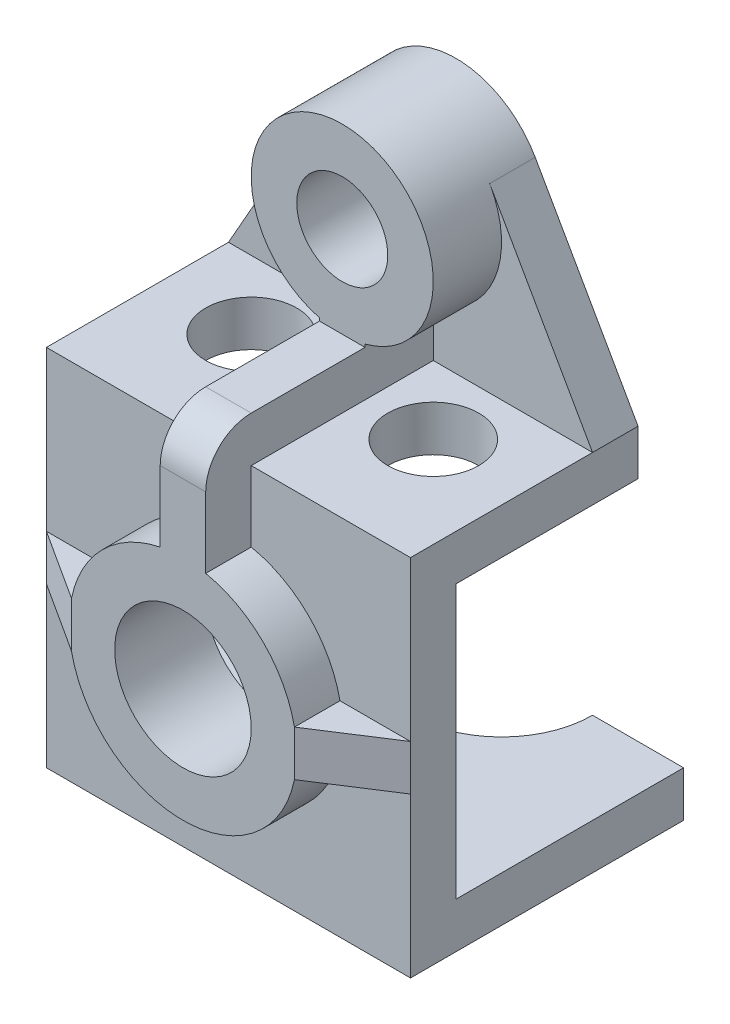
ISO-10303-21;
HEADER;
FILE_DESCRIPTION(('STEP AP214'),'2;1');
FILE_NAME('part.step','',(''),(''),'','','');
FILE_SCHEMA(('AUTOMOTIVE_DESIGN { 1 0 10303 214 1 1 1 1 }'));
ENDSEC;
DATA;
#1=APPLICATION_CONTEXT('core data for automotive mechanical design processes');
#2=APPLICATION_PROTOCOL_DEFINITION('international standard','automotive_design',2000,#1);
#3=PRODUCT_CONTEXT('',#1,'mechanical');
#4=PRODUCT('Part','Part','',(#3));
#5=PRODUCT_RELATED_PRODUCT_CATEGORY('part','',(#4));
#6=PRODUCT_DEFINITION_FORMATION('','',#4);
#7=PRODUCT_DEFINITION_CONTEXT('part definition',#1,'design');
#8=PRODUCT_DEFINITION('design','',#6,#7);
#9=PRODUCT_DEFINITION_SHAPE('','',#8);
#10=(LENGTH_UNIT() NAMED_UNIT(*) SI_UNIT(.MILLI.,.METRE.));
#11=(NAMED_UNIT(*) PLANE_ANGLE_UNIT() SI_UNIT($,.RADIAN.));
#12=(NAMED_UNIT(*) SI_UNIT($,.STERADIAN.) SOLID_ANGLE_UNIT());
#13=UNCERTAINTY_MEASURE_WITH_UNIT(LENGTH_MEASURE(1.E-05),#10,'distance_accuracy_value','');
#14=(GEOMETRIC_REPRESENTATION_CONTEXT(3) GLOBAL_UNCERTAINTY_ASSIGNED_CONTEXT((#13)) GLOBAL_UNIT_ASSIGNED_CONTEXT((#10,
#11,#12)) REPRESENTATION_CONTEXT('',''));
#15=CARTESIAN_POINT('',(0.,0.,0.));
#16=DIRECTION('',(0.,0.,1.));
#17=DIRECTION('',(1.,0.,0.));
#18=AXIS2_PLACEMENT_3D('',#15,#16,#17);
#19=CARTESIAN_POINT('',(40.,0.,-60.));
#20=DIRECTION('',(0.,0.,1.));
#21=DIRECTION('',(1.,0.,0.));
#22=AXIS2_PLACEMENT_3D('',#19,#20,#21);
#23=PLANE('',#22);
#24=DIRECTION('',(0.,1.,0.));
#25=VECTOR('',#24,1.);
#26=CARTESIAN_POINT('',(20.,-0.000999999999999265,-60.));
#27=LINE('',#26,#25);
#28=CARTESIAN_POINT('',(20.,10.,-60.));
#29=VERTEX_POINT('',#28);
#30=CARTESIAN_POINT('',(20.,0.,-60.));
#31=VERTEX_POINT('',#30);
#32=EDGE_CURVE('E226',#29,#31,#27,.F.);
#33=ORIENTED_EDGE('',*,*,#32,.F.);
#34=DIRECTION('',(-1.,0.,0.));
#35=VECTOR('',#34,1.);
#36=CARTESIAN_POINT('',(40.,10.,-60.));
#37=LINE('',#36,#35);
#38=CARTESIAN_POINT('',(40.,10.,-60.));
#39=VERTEX_POINT('',#38);
#40=EDGE_CURVE('E237',#39,#29,#37,.T.);
#41=ORIENTED_EDGE('',*,*,#40,.F.);
#42=DIRECTION('',(0.,1.,0.));
#43=VECTOR('',#42,1.);
#44=CARTESIAN_POINT('',(40.,0.,-60.));
#45=LINE('',#44,#43);
#46=CARTESIAN_POINT('',(40.,0.,-60.));
#47=VERTEX_POINT('',#46);
#48=EDGE_CURVE('E388',#47,#39,#45,.T.);
#49=ORIENTED_EDGE('',*,*,#48,.F.);
#50=DIRECTION('',(-1.,0.,0.));
#51=VECTOR('',#50,1.);
#52=CARTESIAN_POINT('',(40.,0.,-60.));
#53=LINE('',#52,#51);
#54=EDGE_CURVE('E245',#47,#31,#53,.T.);
#55=ORIENTED_EDGE('',*,*,#54,.T.);
#56=EDGE_LOOP('',(#33,#41,#49,#55));
#57=FACE_BOUND('',#56,.T.);
#58=ADVANCED_FACE('F43',(#57),#23,.F.);
#59=DIRECTION('',(0.,1.,0.));
#60=VECTOR('',#59,1.);
#61=CARTESIAN_POINT('',(-20.,-0.000999999999999265,-60.));
#62=LINE('',#61,#60);
#63=CARTESIAN_POINT('',(-20.,0.,-60.));
#64=VERTEX_POINT('',#63);
#65=CARTESIAN_POINT('',(-20.,10.,-60.));
#66=VERTEX_POINT('',#65);
#67=EDGE_CURVE('E59',#64,#66,#62,.T.);
#68=ORIENTED_EDGE('',*,*,#67,.F.);
#69=CARTESIAN_POINT('',(-40.,0.,-60.));
#70=VERTEX_POINT('',#69);
#71=EDGE_CURVE('E250',#64,#70,#53,.T.);
#72=ORIENTED_EDGE('',*,*,#71,.T.);
#73=DIRECTION('',(0.,1.,0.));
#74=VECTOR('',#73,1.);
#75=CARTESIAN_POINT('',(-40.,0.,-60.));
#76=LINE('',#75,#74);
#77=CARTESIAN_POINT('',(-40.,10.,-60.));
#78=VERTEX_POINT('',#77);
#79=EDGE_CURVE('E408',#70,#78,#76,.T.);
#80=ORIENTED_EDGE('',*,*,#79,.T.);
#81=EDGE_CURVE('E247',#66,#78,#37,.T.);
#82=ORIENTED_EDGE('',*,*,#81,.F.);
#83=EDGE_LOOP('',(#68,#72,#80,#82));
#84=FACE_BOUND('',#83,.T.);
#85=ADVANCED_FACE('F588',(#84),#23,.F.);
#86=CARTESIAN_POINT('',(40.,0.,0.));
#87=DIRECTION('',(0.,1.,0.));
#88=DIRECTION('',(0.,0.,1.));
#89=AXIS2_PLACEMENT_3D('',#86,#87,#88);
#90=PLANE('',#89);
#91=CARTESIAN_POINT('',(0.,0.,-60.));
#92=DIRECTION('',(0.,1.,0.));
#93=DIRECTION('',(0.,0.,1.));
#94=AXIS2_PLACEMENT_3D('',#91,#92,#93);
#95=CIRCLE('',#94,20.);
#96=EDGE_CURVE('E231',#31,#64,#95,.F.);
#97=ORIENTED_EDGE('',*,*,#96,.F.);
#98=ORIENTED_EDGE('',*,*,#54,.F.);
#99=DIRECTION('',(0.,0.,-1.));
#100=VECTOR('',#99,1.);
#101=CARTESIAN_POINT('',(40.,0.,0.));
#102=LINE('',#101,#100);
#103=CARTESIAN_POINT('',(40.,0.,0.));
#104=VERTEX_POINT('',#103);
#105=EDGE_CURVE('E384',#104,#47,#102,.T.);
#106=ORIENTED_EDGE('',*,*,#105,.F.);
#107=DIRECTION('',(-1.,0.,0.));
#108=VECTOR('',#107,1.);
#109=CARTESIAN_POINT('',(40.,0.,0.));
#110=LINE('',#109,#108);
#111=CARTESIAN_POINT('',(-40.,0.,0.));
#112=VERTEX_POINT('',#111);
#113=EDGE_CURVE('E253',#104,#112,#110,.T.);
#114=ORIENTED_EDGE('',*,*,#113,.T.);
#115=DIRECTION('',(0.,0.,-1.));
#116=VECTOR('',#115,1.);
#117=CARTESIAN_POINT('',(-40.,0.,0.));
#118=LINE('',#117,#116);
#119=EDGE_CURVE('E401',#112,#70,#118,.T.);
#120=ORIENTED_EDGE('',*,*,#119,.T.);
#121=ORIENTED_EDGE('',*,*,#71,.F.);
#122=EDGE_LOOP('',(#97,#98,#106,#114,#120,#121));
#123=FACE_BOUND('',#122,.T.);
#124=ADVANCED_FACE('F457',(#123),#90,.F.);
#125=CARTESIAN_POINT('',(40.,10.,-10.));
#126=DIRECTION('',(0.,-1.,0.));
#127=DIRECTION('',(0.,0.,-1.));
#128=AXIS2_PLACEMENT_3D('',#125,#126,#127);
#129=PLANE('',#128);
#130=CARTESIAN_POINT('',(0.,10.,-60.));
#131=DIRECTION('',(0.,1.,0.));
#132=DIRECTION('',(0.,0.,1.));
#133=AXIS2_PLACEMENT_3D('',#130,#131,#132);
#134=CIRCLE('',#133,20.);
#135=EDGE_CURVE('E224',#66,#29,#134,.T.);
#136=ORIENTED_EDGE('',*,*,#135,.F.);
#137=ORIENTED_EDGE('',*,*,#81,.T.);
#138=DIRECTION('',(0.,0.,1.));
#139=VECTOR('',#138,1.);
#140=CARTESIAN_POINT('',(-40.,10.,-10.));
#141=LINE('',#140,#139);
#142=CARTESIAN_POINT('',(-40.,10.,-10.));
#143=VERTEX_POINT('',#142);
#144=EDGE_CURVE('E410',#78,#143,#141,.T.);
#145=ORIENTED_EDGE('',*,*,#144,.T.);
#146=DIRECTION('',(-1.,0.,0.));
#147=VECTOR('',#146,1.);
#148=CARTESIAN_POINT('',(40.,10.,-10.));
#149=LINE('',#148,#147);
#150=CARTESIAN_POINT('',(40.,10.,-10.));
#151=VERTEX_POINT('',#150);
#152=EDGE_CURVE('E252',#151,#143,#149,.T.);
#153=ORIENTED_EDGE('',*,*,#152,.F.);
#154=DIRECTION('',(0.,0.,1.));
#155=VECTOR('',#154,1.);
#156=CARTESIAN_POINT('',(40.,10.,-10.));
#157=LINE('',#156,#155);
#158=EDGE_CURVE('E246',#39,#151,#157,.T.);
#159=ORIENTED_EDGE('',*,*,#158,.F.);
#160=ORIENTED_EDGE('',*,*,#40,.T.);
#161=EDGE_LOOP('',(#136,#137,#145,#153,#159,#160));
#162=FACE_BOUND('',#161,.T.);
#163=ADVANCED_FACE('F242',(#162),#129,.F.);
#164=CARTESIAN_POINT('',(0.,45.,0.));
#165=DIRECTION('',(0.,1.,0.));
#166=DIRECTION('',(-1.,0.,0.));
#167=AXIS2_PLACEMENT_3D('',#164,#165,#166);
#168=PLANE('',#167);
#169=DIRECTION('',(0.840377920149043,0.,0.542000877606272));
#170=VECTOR('',#169,1.);
#171=CARTESIAN_POINT('',(-24.4948974278318,45.,10.));
#172=LINE('',#171,#170);
#173=CARTESIAN_POINT('',(-40.,45.,0.));
#174=VERTEX_POINT('',#173);
#175=CARTESIAN_POINT('',(-24.4948974278318,45.,10.));
#176=VERTEX_POINT('',#175);
#177=EDGE_CURVE('E472',#174,#176,#172,.T.);
#178=ORIENTED_EDGE('',*,*,#177,.T.);
#179=DIRECTION('',(0.,0.,-1.));
#180=VECTOR('',#179,1.);
#181=CARTESIAN_POINT('',(-24.4948974278318,45.,10.));
#182=LINE('',#181,#180);
#183=CARTESIAN_POINT('',(-24.4948974278318,45.,0.));
#184=VERTEX_POINT('',#183);
#185=EDGE_CURVE('E490',#184,#176,#182,.F.);
#186=ORIENTED_EDGE('',*,*,#185,.F.);
#187=DIRECTION('',(1.,0.,0.));
#188=VECTOR('',#187,1.);
#189=CARTESIAN_POINT('',(40.,45.,0.));
#190=LINE('',#189,#188);
#191=EDGE_CURVE('E487',#174,#184,#190,.T.);
#192=ORIENTED_EDGE('',*,*,#191,.F.);
#193=EDGE_LOOP('',(#178,#186,#192));
#194=FACE_BOUND('',#193,.T.);
#195=ADVANCED_FACE('F660',(#194),#168,.T.);
#196=CARTESIAN_POINT('',(0.,35.,0.));
#197=DIRECTION('',(0.,1.,0.));
#198=DIRECTION('',(-1.,0.,0.));
#199=AXIS2_PLACEMENT_3D('',#196,#197,#198);
#200=PLANE('',#199);
#201=DIRECTION('',(0.,0.,-1.));
#202=VECTOR('',#201,1.);
#203=CARTESIAN_POINT('',(-24.4948974278318,35.,10.));
#204=LINE('',#203,#202);
#205=CARTESIAN_POINT('',(-24.4948974278318,35.,0.));
#206=VERTEX_POINT('',#205);
#207=CARTESIAN_POINT('',(-24.4948974278318,35.,10.));
#208=VERTEX_POINT('',#207);
#209=EDGE_CURVE('E69',#206,#208,#204,.F.);
#210=ORIENTED_EDGE('',*,*,#209,.T.);
#211=DIRECTION('',(-0.840377920149043,0.,-0.542000877606272));
#212=VECTOR('',#211,1.);
#213=CARTESIAN_POINT('',(-24.4948974278318,35.,10.));
#214=LINE('',#213,#212);
#215=CARTESIAN_POINT('',(-40.,35.,0.));
#216=VERTEX_POINT('',#215);
#217=EDGE_CURVE('E481',#208,#216,#214,.T.);
#218=ORIENTED_EDGE('',*,*,#217,.T.);
#219=DIRECTION('',(1.,0.,0.));
#220=VECTOR('',#219,1.);
#221=CARTESIAN_POINT('',(40.,35.,0.));
#222=LINE('',#221,#220);
#223=EDGE_CURVE('E495',#216,#206,#222,.T.);
#224=ORIENTED_EDGE('',*,*,#223,.T.);
#225=EDGE_LOOP('',(#210,#218,#224));
#226=FACE_BOUND('',#225,.T.);
#227=ADVANCED_FACE('F548',(#226),#200,.F.);
#228=CARTESIAN_POINT('',(0.,40.,10.));
#229=DIRECTION('',(0.,0.,-1.));
#230=DIRECTION('',(-1.,0.,0.));
#231=AXIS2_PLACEMENT_3D('',#228,#229,#230);
#232=CYLINDRICAL_SURFACE('',#231,25.);
#233=CARTESIAN_POINT('',(0.,40.,10.));
#234=DIRECTION('',(0.,0.,1.));
#235=DIRECTION('',(1.,0.,0.));
#236=AXIS2_PLACEMENT_3D('',#233,#234,#235);
#237=CIRCLE('',#236,25.);
#238=CARTESIAN_POINT('',(24.4948974278318,35.,10.));
#239=VERTEX_POINT('',#238);
#240=EDGE_CURVE('E339',#208,#239,#237,.T.);
#241=ORIENTED_EDGE('',*,*,#240,.F.);
#242=ORIENTED_EDGE('',*,*,#209,.F.);
#243=CARTESIAN_POINT('',(0.,40.,0.));
#244=DIRECTION('',(0.,0.,1.));
#245=DIRECTION('',(1.,0.,0.));
#246=AXIS2_PLACEMENT_3D('',#243,#244,#245);
#247=CIRCLE('',#246,25.);
#248=CARTESIAN_POINT('',(24.4948974278318,35.,0.));
#249=VERTEX_POINT('',#248);
#250=EDGE_CURVE('E344',#206,#249,#247,.T.);
#251=ORIENTED_EDGE('',*,*,#250,.T.);
#252=DIRECTION('',(0.,0.,-1.));
#253=VECTOR('',#252,1.);
#254=CARTESIAN_POINT('',(24.4948974278318,35.,10.));
#255=LINE('',#254,#253);
#256=EDGE_CURVE('E512',#239,#249,#255,.T.);
#257=ORIENTED_EDGE('',*,*,#256,.F.);
#258=EDGE_LOOP('',(#241,#242,#251,#257));
#259=FACE_BOUND('',#258,.T.);
#260=ADVANCED_FACE('F552',(#259),#232,.T.);
#261=ORIENTED_EDGE('',*,*,#185,.T.);
#262=CARTESIAN_POINT('',(-5.,64.4948974278318,10.));
#263=VERTEX_POINT('',#262);
#264=EDGE_CURVE('E337',#263,#176,#237,.T.);
#265=ORIENTED_EDGE('',*,*,#264,.F.);
#266=DIRECTION('',(0.,0.,-1.));
#267=VECTOR('',#266,1.);
#268=CARTESIAN_POINT('',(-5.,64.4948974278318,10.));
#269=LINE('',#268,#267);
#270=CARTESIAN_POINT('',(-5.,64.4948974278318,0.));
#271=VERTEX_POINT('',#270);
#272=EDGE_CURVE('E261',#271,#263,#269,.F.);
#273=ORIENTED_EDGE('',*,*,#272,.F.);
#274=EDGE_CURVE('E265',#271,#184,#247,.T.);
#275=ORIENTED_EDGE('',*,*,#274,.T.);
#276=EDGE_LOOP('',(#261,#265,#273,#275));
#277=FACE_BOUND('',#276,.T.);
#278=ADVANCED_FACE('F544',(#277),#232,.T.);
#279=CARTESIAN_POINT('',(40.,0.,0.));
#280=DIRECTION('',(0.,0.,-1.));
#281=DIRECTION('',(-1.,0.,0.));
#282=AXIS2_PLACEMENT_3D('',#279,#280,#281);
#283=PLANE('',#282);
#284=ORIENTED_EDGE('',*,*,#223,.F.);
#285=DIRECTION('',(0.,-1.,0.));
#286=VECTOR('',#285,1.);
#287=CARTESIAN_POINT('',(-40.,0.,0.));
#288=LINE('',#287,#286);
#289=EDGE_CURVE('E380',#216,#112,#288,.T.);
#290=ORIENTED_EDGE('',*,*,#289,.T.);
#291=ORIENTED_EDGE('',*,*,#113,.F.);
#292=DIRECTION('',(0.,-1.,0.));
#293=VECTOR('',#292,1.);
#294=CARTESIAN_POINT('',(40.,0.,0.));
#295=LINE('',#294,#293);
#296=CARTESIAN_POINT('',(40.,35.,0.));
#297=VERTEX_POINT('',#296);
#298=EDGE_CURVE('E381',#297,#104,#295,.T.);
#299=ORIENTED_EDGE('',*,*,#298,.F.);
#300=DIRECTION('',(1.,0.,0.));
#301=VECTOR('',#300,1.);
#302=CARTESIAN_POINT('',(40.,35.,0.));
#303=LINE('',#302,#301);
#304=EDGE_CURVE('E511',#249,#297,#303,.T.);
#305=ORIENTED_EDGE('',*,*,#304,.F.);
#306=ORIENTED_EDGE('',*,*,#250,.F.);
#307=EDGE_LOOP('',(#284,#290,#291,#299,#305,#306));
#308=FACE_BOUND('',#307,.T.);
#309=ADVANCED_FACE('F603',(#308),#283,.F.);
#310=CARTESIAN_POINT('',(0.,35.,0.));
#311=DIRECTION('',(0.,1.,0.));
#312=DIRECTION('',(1.,0.,0.));
#313=AXIS2_PLACEMENT_3D('',#310,#311,#312);
#314=PLANE('',#313);
#315=DIRECTION('',(0.840377920149043,0.,-0.542000877606272));
#316=VECTOR('',#315,1.);
#317=CARTESIAN_POINT('',(24.4948974278318,35.,10.));
#318=LINE('',#317,#316);
#319=EDGE_CURVE('E496',#239,#297,#318,.T.);
#320=ORIENTED_EDGE('',*,*,#319,.F.);
#321=ORIENTED_EDGE('',*,*,#256,.T.);
#322=ORIENTED_EDGE('',*,*,#304,.T.);
#323=EDGE_LOOP('',(#320,#321,#322));
#324=FACE_BOUND('',#323,.T.);
#325=ADVANCED_FACE('F607',(#324),#314,.F.);
#326=CARTESIAN_POINT('',(0.,45.,0.));
#327=DIRECTION('',(0.,1.,0.));
#328=DIRECTION('',(1.,0.,0.));
#329=AXIS2_PLACEMENT_3D('',#326,#327,#328);
#330=PLANE('',#329);
#331=DIRECTION('',(0.,0.,-1.));
#332=VECTOR('',#331,1.);
#333=CARTESIAN_POINT('',(24.4948974278318,45.,10.));
#334=LINE('',#333,#332);
#335=CARTESIAN_POINT('',(24.4948974278318,45.,10.));
#336=VERTEX_POINT('',#335);
#337=CARTESIAN_POINT('',(24.4948974278318,45.,0.));
#338=VERTEX_POINT('',#337);
#339=EDGE_CURVE('E504',#336,#338,#334,.T.);
#340=ORIENTED_EDGE('',*,*,#339,.F.);
#341=DIRECTION('',(-0.840377920149043,0.,0.542000877606272));
#342=VECTOR('',#341,1.);
#343=CARTESIAN_POINT('',(24.4948974278318,45.,10.));
#344=LINE('',#343,#342);
#345=CARTESIAN_POINT('',(40.,45.,0.));
#346=VERTEX_POINT('',#345);
#347=EDGE_CURVE('E498',#346,#336,#344,.T.);
#348=ORIENTED_EDGE('',*,*,#347,.F.);
#349=DIRECTION('',(1.,0.,0.));
#350=VECTOR('',#349,1.);
#351=CARTESIAN_POINT('',(40.,45.,0.));
#352=LINE('',#351,#350);
#353=EDGE_CURVE('E507',#338,#346,#352,.T.);
#354=ORIENTED_EDGE('',*,*,#353,.F.);
#355=EDGE_LOOP('',(#340,#348,#354));
#356=FACE_BOUND('',#355,.T.);
#357=ADVANCED_FACE('F648',(#356),#330,.T.);
#358=CARTESIAN_POINT('',(0.,40.,10.));
#359=DIRECTION('',(0.,0.,1.));
#360=DIRECTION('',(1.,0.,0.));
#361=AXIS2_PLACEMENT_3D('',#358,#359,#360);
#362=PLANE('',#361);
#363=ORIENTED_EDGE('',*,*,#264,.T.);
#364=DIRECTION('',(0.,1.,0.));
#365=VECTOR('',#364,1.);
#366=CARTESIAN_POINT('',(-24.4948974278318,-0.001000000000001,10.));
#367=LINE('',#366,#365);
#368=EDGE_CURVE('E478',#208,#176,#367,.T.);
#369=ORIENTED_EDGE('',*,*,#368,.F.);
#370=ORIENTED_EDGE('',*,*,#240,.T.);
#371=DIRECTION('',(0.,1.,0.));
#372=VECTOR('',#371,1.);
#373=CARTESIAN_POINT('',(24.4948974278318,-0.001000000000001,10.));
#374=LINE('',#373,#372);
#375=EDGE_CURVE('E501',#239,#336,#374,.T.);
#376=ORIENTED_EDGE('',*,*,#375,.T.);
#377=CARTESIAN_POINT('',(5.,64.4948974278318,10.));
#378=VERTEX_POINT('',#377);
#379=EDGE_CURVE('E334',#336,#378,#237,.T.);
#380=ORIENTED_EDGE('',*,*,#379,.T.);
#381=DIRECTION('',(0.,-1.,0.));
#382=VECTOR('',#381,1.);
#383=CARTESIAN_POINT('',(5.,95.,10.));
#384=LINE('',#383,#382);
#385=CARTESIAN_POINT('',(5.,80.,10.));
#386=VERTEX_POINT('',#385);
#387=EDGE_CURVE('E276',#386,#378,#384,.T.);
#388=ORIENTED_EDGE('',*,*,#387,.F.);
#389=DIRECTION('',(1.,0.,0.));
#390=VECTOR('',#389,1.);
#391=CARTESIAN_POINT('',(-5.,80.,10.));
#392=LINE('',#391,#390);
#393=CARTESIAN_POINT('',(-5.,80.,10.));
#394=VERTEX_POINT('',#393);
#395=EDGE_CURVE('E51',#386,#394,#392,.F.);
#396=ORIENTED_EDGE('',*,*,#395,.T.);
#397=DIRECTION('',(0.,-1.,0.));
#398=VECTOR('',#397,1.);
#399=CARTESIAN_POINT('',(-5.,95.,10.));
#400=LINE('',#399,#398);
#401=EDGE_CURVE('E279',#394,#263,#400,.T.);
#402=ORIENTED_EDGE('',*,*,#401,.T.);
#403=EDGE_LOOP('',(#363,#369,#370,#376,#380,#388,#396,#402));
#404=FACE_BOUND('',#403,.T.);
#405=CARTESIAN_POINT('',(0.,40.,10.));
#406=DIRECTION('',(0.,0.,1.));
#407=DIRECTION('',(1.,0.,0.));
#408=AXIS2_PLACEMENT_3D('',#405,#406,#407);
#409=CIRCLE('',#408,15.);
#410=CARTESIAN_POINT('',(15.,40.,10.));
#411=VERTEX_POINT('',#410);
#412=EDGE_CURVE('E335',#411,#411,#409,.T.);
#413=ORIENTED_EDGE('',*,*,#412,.F.);
#414=EDGE_LOOP('',(#413));
#415=FACE_BOUND('',#414,.T.);
#416=ADVANCED_FACE('F273',(#404,#415),#362,.T.);
#417=CARTESIAN_POINT('',(24.4948974278318,-0.001000000000001,10.));
#418=DIRECTION('',(-0.542000877606272,0.,-0.840377920149043));
#419=DIRECTION('',(-0.840377920149043,0.,0.542000877606272));
#420=AXIS2_PLACEMENT_3D('',#417,#418,#419);
#421=PLANE('',#420);
#422=ORIENTED_EDGE('',*,*,#375,.F.);
#423=ORIENTED_EDGE('',*,*,#319,.T.);
#424=DIRECTION('',(0.,1.,0.));
#425=VECTOR('',#424,1.);
#426=CARTESIAN_POINT('',(40.,35.,0.));
#427=LINE('',#426,#425);
#428=EDGE_CURVE('E503',#297,#346,#427,.T.);
#429=ORIENTED_EDGE('',*,*,#428,.T.);
#430=ORIENTED_EDGE('',*,*,#347,.T.);
#431=EDGE_LOOP('',(#422,#423,#429,#430));
#432=FACE_BOUND('',#431,.T.);
#433=ADVANCED_FACE('F620',(#432),#421,.F.);
#434=ORIENTED_EDGE('',*,*,#379,.F.);
#435=ORIENTED_EDGE('',*,*,#339,.T.);
#436=CARTESIAN_POINT('',(5.,64.4948974278318,0.));
#437=VERTEX_POINT('',#436);
#438=EDGE_CURVE('E257',#338,#437,#247,.T.);
#439=ORIENTED_EDGE('',*,*,#438,.T.);
#440=DIRECTION('',(0.,0.,-1.));
#441=VECTOR('',#440,1.);
#442=CARTESIAN_POINT('',(5.,64.4948974278318,10.));
#443=LINE('',#442,#441);
#444=EDGE_CURVE('E260',#378,#437,#443,.T.);
#445=ORIENTED_EDGE('',*,*,#444,.F.);
#446=EDGE_LOOP('',(#434,#435,#439,#445));
#447=FACE_BOUND('',#446,.T.);
#448=ADVANCED_FACE('F558',(#447),#232,.T.);
#449=CARTESIAN_POINT('',(-40.,80.,0.));
#450=VERTEX_POINT('',#449);
#451=EDGE_CURVE('E399',#450,#174,#288,.T.);
#452=ORIENTED_EDGE('',*,*,#451,.T.);
#453=ORIENTED_EDGE('',*,*,#191,.T.);
#454=ORIENTED_EDGE('',*,*,#274,.F.);
#455=DIRECTION('',(0.,1.,0.));
#456=VECTOR('',#455,1.);
#457=CARTESIAN_POINT('',(-5.,66.4615998768807,0.));
#458=LINE('',#457,#456);
#459=CARTESIAN_POINT('',(-5.,80.,0.));
#460=VERTEX_POINT('',#459);
#461=EDGE_CURVE('E304',#271,#460,#458,.T.);
#462=ORIENTED_EDGE('',*,*,#461,.T.);
#463=DIRECTION('',(-1.,0.,0.));
#464=VECTOR('',#463,1.);
#465=CARTESIAN_POINT('',(40.,80.,0.));
#466=LINE('',#465,#464);
#467=EDGE_CURVE('E398',#460,#450,#466,.T.);
#468=ORIENTED_EDGE('',*,*,#467,.T.);
#469=EDGE_LOOP('',(#452,#453,#454,#462,#468));
#470=FACE_BOUND('',#469,.T.);
#471=ADVANCED_FACE('F539',(#470),#283,.F.);
#472=CARTESIAN_POINT('',(-5.,95.,-40.));
#473=DIRECTION('',(1.,0.,0.));
#474=DIRECTION('',(0.,0.,-1.));
#475=AXIS2_PLACEMENT_3D('',#472,#473,#474);
#476=PLANE('',#475);
#477=ORIENTED_EDGE('',*,*,#401,.F.);
#478=CARTESIAN_POINT('',(-5.,80.,0.));
#479=DIRECTION('',(1.,0.,0.));
#480=DIRECTION('',(0.,0.,-1.));
#481=AXIS2_PLACEMENT_3D('',#478,#479,#480);
#482=CIRCLE('',#481,10.);
#483=CARTESIAN_POINT('',(-5.,90.,0.));
#484=VERTEX_POINT('',#483);
#485=EDGE_CURVE('E11',#394,#484,#482,.F.);
#486=ORIENTED_EDGE('',*,*,#485,.T.);
#487=DIRECTION('',(0.,0.,1.));
#488=VECTOR('',#487,1.);
#489=CARTESIAN_POINT('',(-5.,90.,-25.));
#490=LINE('',#489,#488);
#491=CARTESIAN_POINT('',(-5.,90.,-25.));
#492=VERTEX_POINT('',#491);
#493=EDGE_CURVE('E300',#492,#484,#490,.T.);
#494=ORIENTED_EDGE('',*,*,#493,.F.);
#495=DIRECTION('',(0.,-1.,0.));
#496=VECTOR('',#495,1.);
#497=CARTESIAN_POINT('',(-5.,0.,-25.));
#498=LINE('',#497,#496);
#499=CARTESIAN_POINT('',(-5.,90.6350832689629,-25.));
#500=VERTEX_POINT('',#499);
#501=EDGE_CURVE('E519',#500,#492,#498,.T.);
#502=ORIENTED_EDGE('',*,*,#501,.F.);
#503=DIRECTION('',(0.,0.,-1.));
#504=VECTOR('',#503,1.);
#505=CARTESIAN_POINT('',(-5.,90.6350832689629,-25.));
#506=LINE('',#505,#504);
#507=CARTESIAN_POINT('',(-5.,90.6350832689629,-40.));
#508=VERTEX_POINT('',#507);
#509=EDGE_CURVE('E329',#508,#500,#506,.F.);
#510=ORIENTED_EDGE('',*,*,#509,.F.);
#511=DIRECTION('',(0.,-1.,0.));
#512=VECTOR('',#511,1.);
#513=CARTESIAN_POINT('',(-5.,95.,-40.));
#514=LINE('',#513,#512);
#515=CARTESIAN_POINT('',(-5.,80.,-40.));
#516=VERTEX_POINT('',#515);
#517=EDGE_CURVE('E287',#508,#516,#514,.T.);
#518=ORIENTED_EDGE('',*,*,#517,.T.);
#519=DIRECTION('',(0.,0.,-1.));
#520=VECTOR('',#519,1.);
#521=CARTESIAN_POINT('',(-5.,80.,0.));
#522=LINE('',#521,#520);
#523=EDGE_CURVE('E312',#460,#516,#522,.T.);
#524=ORIENTED_EDGE('',*,*,#523,.F.);
#525=ORIENTED_EDGE('',*,*,#461,.F.);
#526=ORIENTED_EDGE('',*,*,#272,.T.);
#527=EDGE_LOOP('',(#477,#486,#494,#502,#510,#518,#524,#525,#526));
#528=FACE_BOUND('',#527,.T.);
#529=ADVANCED_FACE('F283',(#528),#476,.F.);
#530=CARTESIAN_POINT('',(5.,95.,10.));
#531=DIRECTION('',(-1.,0.,0.));
#532=DIRECTION('',(0.,0.,1.));
#533=AXIS2_PLACEMENT_3D('',#530,#531,#532);
#534=PLANE('',#533);
#535=DIRECTION('',(0.,0.,-1.));
#536=VECTOR('',#535,1.);
#537=CARTESIAN_POINT('',(5.,90.,-25.));
#538=LINE('',#537,#536);
#539=CARTESIAN_POINT('',(5.,90.,0.));
#540=VERTEX_POINT('',#539);
#541=CARTESIAN_POINT('',(5.,90.,-25.));
#542=VERTEX_POINT('',#541);
#543=EDGE_CURVE('E294',#540,#542,#538,.T.);
#544=ORIENTED_EDGE('',*,*,#543,.F.);
#545=CARTESIAN_POINT('',(5.,80.,0.));
#546=DIRECTION('',(-1.,0.,0.));
#547=DIRECTION('',(0.,0.,1.));
#548=AXIS2_PLACEMENT_3D('',#545,#546,#547);
#549=CIRCLE('',#548,10.);
#550=EDGE_CURVE('E268',#540,#386,#549,.F.);
#551=ORIENTED_EDGE('',*,*,#550,.T.);
#552=ORIENTED_EDGE('',*,*,#387,.T.);
#553=ORIENTED_EDGE('',*,*,#444,.T.);
#554=DIRECTION('',(0.,1.,0.));
#555=VECTOR('',#554,1.);
#556=CARTESIAN_POINT('',(5.,66.4615998768807,0.));
#557=LINE('',#556,#555);
#558=CARTESIAN_POINT('',(5.,80.,0.));
#559=VERTEX_POINT('',#558);
#560=EDGE_CURVE('E309',#437,#559,#557,.T.);
#561=ORIENTED_EDGE('',*,*,#560,.T.);
#562=DIRECTION('',(0.,0.,-1.));
#563=VECTOR('',#562,1.);
#564=CARTESIAN_POINT('',(5.,80.,0.));
#565=LINE('',#564,#563);
#566=CARTESIAN_POINT('',(5.,80.,-40.));
#567=VERTEX_POINT('',#566);
#568=EDGE_CURVE('E315',#559,#567,#565,.T.);
#569=ORIENTED_EDGE('',*,*,#568,.T.);
#570=DIRECTION('',(0.,-1.,0.));
#571=VECTOR('',#570,1.);
#572=CARTESIAN_POINT('',(5.,95.,-40.));
#573=LINE('',#572,#571);
#574=CARTESIAN_POINT('',(5.,90.6350832689629,-40.));
#575=VERTEX_POINT('',#574);
#576=EDGE_CURVE('E317',#575,#567,#573,.T.);
#577=ORIENTED_EDGE('',*,*,#576,.F.);
#578=DIRECTION('',(0.,0.,-1.));
#579=VECTOR('',#578,1.);
#580=CARTESIAN_POINT('',(5.,90.6350832689629,-25.));
#581=LINE('',#580,#579);
#582=CARTESIAN_POINT('',(5.,90.6350832689629,-25.));
#583=VERTEX_POINT('',#582);
#584=EDGE_CURVE('E322',#583,#575,#581,.T.);
#585=ORIENTED_EDGE('',*,*,#584,.F.);
#586=DIRECTION('',(0.,1.,0.));
#587=VECTOR('',#586,1.);
#588=CARTESIAN_POINT('',(5.,95.,-25.));
#589=LINE('',#588,#587);
#590=EDGE_CURVE('E305',#542,#583,#589,.T.);
#591=ORIENTED_EDGE('',*,*,#590,.F.);
#592=EDGE_LOOP('',(#544,#551,#552,#553,#561,#569,#577,#585,#591));
#593=FACE_BOUND('',#592,.T.);
#594=ADVANCED_FACE('F297',(#593),#534,.F.);
#595=ORIENTED_EDGE('',*,*,#438,.F.);
#596=ORIENTED_EDGE('',*,*,#353,.T.);
#597=CARTESIAN_POINT('',(40.,80.,0.));
#598=VERTEX_POINT('',#597);
#599=EDGE_CURVE('E379',#598,#346,#295,.T.);
#600=ORIENTED_EDGE('',*,*,#599,.F.);
#601=EDGE_CURVE('E423',#598,#559,#466,.T.);
#602=ORIENTED_EDGE('',*,*,#601,.T.);
#603=ORIENTED_EDGE('',*,*,#560,.F.);
#604=EDGE_LOOP('',(#595,#596,#600,#602,#603));
#605=FACE_BOUND('',#604,.T.);
#606=ADVANCED_FACE('F561',(#605),#283,.F.);
#607=CARTESIAN_POINT('',(0.,0.,-40.));
#608=DIRECTION('',(0.,0.,-1.));
#609=DIRECTION('',(-1.,0.,0.));
#610=AXIS2_PLACEMENT_3D('',#607,#608,#609);
#611=PLANE('',#610);
#612=ORIENTED_EDGE('',*,*,#576,.T.);
#613=DIRECTION('',(1.,0.,0.));
#614=VECTOR('',#613,1.);
#615=CARTESIAN_POINT('',(0.,80.,-40.));
#616=LINE('',#615,#614);
#617=CARTESIAN_POINT('',(40.,80.,-40.));
#618=VERTEX_POINT('',#617);
#619=EDGE_CURVE('E360',#567,#618,#616,.T.);
#620=ORIENTED_EDGE('',*,*,#619,.T.);
#621=DIRECTION('',(-0.493212111192935,0.869909083394701,0.));
#622=VECTOR('',#621,1.);
#623=CARTESIAN_POINT('',(64.5936481802652,36.6226427528718,-40.));
#624=LINE('',#623,#622);
#625=CARTESIAN_POINT('',(17.398181667894,119.864242223859,-40.));
#626=VERTEX_POINT('',#625);
#627=EDGE_CURVE('E366',#618,#626,#624,.T.);
#628=ORIENTED_EDGE('',*,*,#627,.T.);
#629=CARTESIAN_POINT('',(0.,110.,-40.));
#630=DIRECTION('',(0.,0.,-1.));
#631=DIRECTION('',(-1.,0.,0.));
#632=AXIS2_PLACEMENT_3D('',#629,#630,#631);
#633=CIRCLE('',#632,20.);
#634=EDGE_CURVE('E361',#626,#575,#633,.T.);
#635=ORIENTED_EDGE('',*,*,#634,.T.);
#636=EDGE_LOOP('',(#612,#620,#628,#635));
#637=FACE_BOUND('',#636,.T.);
#638=ADVANCED_FACE('F569',(#637),#611,.F.);
#639=CARTESIAN_POINT('',(40.,80.,0.));
#640=DIRECTION('',(0.,-1.,0.));
#641=DIRECTION('',(0.,0.,-1.));
#642=AXIS2_PLACEMENT_3D('',#639,#640,#641);
#643=PLANE('',#642);
#644=CARTESIAN_POINT('',(-20.,80.,-25.));
#645=DIRECTION('',(0.,1.,0.));
#646=DIRECTION('',(0.,0.,1.));
#647=AXIS2_PLACEMENT_3D('',#644,#645,#646);
#648=CIRCLE('',#647,10.);
#649=CARTESIAN_POINT('',(-20.,80.,-15.));
#650=VERTEX_POINT('',#649);
#651=EDGE_CURVE('E473',#650,#650,#648,.T.);
#652=ORIENTED_EDGE('',*,*,#651,.F.);
#653=EDGE_LOOP('',(#652));
#654=FACE_BOUND('',#653,.T.);
#655=ORIENTED_EDGE('',*,*,#523,.T.);
#656=CARTESIAN_POINT('',(-40.,80.,-40.));
#657=VERTEX_POINT('',#656);
#658=EDGE_CURVE('E354',#657,#516,#616,.T.);
#659=ORIENTED_EDGE('',*,*,#658,.F.);
#660=DIRECTION('',(0.,0.,1.));
#661=VECTOR('',#660,1.);
#662=CARTESIAN_POINT('',(-40.,80.,0.));
#663=LINE('',#662,#661);
#664=EDGE_CURVE('E420',#657,#450,#663,.T.);
#665=ORIENTED_EDGE('',*,*,#664,.T.);
#666=ORIENTED_EDGE('',*,*,#467,.F.);
#667=EDGE_LOOP('',(#655,#659,#665,#666));
#668=FACE_BOUND('',#667,.T.);
#669=ADVANCED_FACE('F531',(#654,#668),#643,.F.);
#670=ORIENTED_EDGE('',*,*,#658,.T.);
#671=ORIENTED_EDGE('',*,*,#517,.F.);
#672=CARTESIAN_POINT('',(-17.398181667894,119.864242223859,-40.));
#673=VERTEX_POINT('',#672);
#674=EDGE_CURVE('E365',#508,#673,#633,.T.);
#675=ORIENTED_EDGE('',*,*,#674,.T.);
#676=DIRECTION('',(0.493212111192935,0.869909083394701,0.));
#677=VECTOR('',#676,1.);
#678=CARTESIAN_POINT('',(-64.5936481802652,36.6226427528718,-40.));
#679=LINE('',#678,#677);
#680=EDGE_CURVE('E356',#657,#673,#679,.T.);
#681=ORIENTED_EDGE('',*,*,#680,.F.);
#682=EDGE_LOOP('',(#670,#671,#675,#681));
#683=FACE_BOUND('',#682,.T.);
#684=ADVANCED_FACE('F528',(#683),#611,.F.);
#685=CARTESIAN_POINT('',(0.,110.,-25.));
#686=DIRECTION('',(0.,0.,-1.));
#687=DIRECTION('',(-1.,0.,0.));
#688=AXIS2_PLACEMENT_3D('',#685,#686,#687);
#689=CYLINDRICAL_SURFACE('',#688,20.);
#690=ORIENTED_EDGE('',*,*,#674,.F.);
#691=ORIENTED_EDGE('',*,*,#509,.T.);
#692=CARTESIAN_POINT('',(0.,110.,-25.));
#693=DIRECTION('',(0.,0.,-1.));
#694=DIRECTION('',(-1.,0.,0.));
#695=AXIS2_PLACEMENT_3D('',#692,#693,#694);
#696=CIRCLE('',#695,20.);
#697=EDGE_CURVE('E349',#500,#583,#696,.T.);
#698=ORIENTED_EDGE('',*,*,#697,.T.);
#699=ORIENTED_EDGE('',*,*,#584,.T.);
#700=ORIENTED_EDGE('',*,*,#634,.F.);
#701=DIRECTION('',(0.,0.,-1.));
#702=VECTOR('',#701,1.);
#703=CARTESIAN_POINT('',(17.398181667894,119.864242223859,-40.));
#704=LINE('',#703,#702);
#705=CARTESIAN_POINT('',(17.398181667894,119.864242223859,-50.));
#706=VERTEX_POINT('',#705);
#707=EDGE_CURVE('E374',#626,#706,#704,.T.);
#708=ORIENTED_EDGE('',*,*,#707,.T.);
#709=CARTESIAN_POINT('',(0.,110.,-50.));
#710=DIRECTION('',(0.,0.,-1.));
#711=DIRECTION('',(-1.,0.,0.));
#712=AXIS2_PLACEMENT_3D('',#709,#710,#711);
#713=CIRCLE('',#712,20.);
#714=CARTESIAN_POINT('',(-17.398181667894,119.864242223859,-50.));
#715=VERTEX_POINT('',#714);
#716=EDGE_CURVE('E346',#715,#706,#713,.T.);
#717=ORIENTED_EDGE('',*,*,#716,.F.);
#718=DIRECTION('',(0.,0.,-1.));
#719=VECTOR('',#718,1.);
#720=CARTESIAN_POINT('',(-17.398181667894,119.864242223859,-40.));
#721=LINE('',#720,#719);
#722=EDGE_CURVE('E367',#673,#715,#721,.T.);
#723=ORIENTED_EDGE('',*,*,#722,.F.);
#724=EDGE_LOOP('',(#690,#691,#698,#699,#700,#708,#717,#723));
#725=FACE_BOUND('',#724,.T.);
#726=ADVANCED_FACE('F522',(#725),#689,.T.);
#727=CARTESIAN_POINT('',(0.,0.,-25.));
#728=DIRECTION('',(0.,0.,-1.));
#729=DIRECTION('',(-1.,0.,0.));
#730=AXIS2_PLACEMENT_3D('',#727,#728,#729);
#731=PLANE('',#730);
#732=ORIENTED_EDGE('',*,*,#697,.F.);
#733=ORIENTED_EDGE('',*,*,#501,.T.);
#734=DIRECTION('',(1.,0.,0.));
#735=VECTOR('',#734,1.);
#736=CARTESIAN_POINT('',(-40.001,90.,-25.));
#737=LINE('',#736,#735);
#738=EDGE_CURVE('E303',#492,#542,#737,.T.);
#739=ORIENTED_EDGE('',*,*,#738,.T.);
#740=ORIENTED_EDGE('',*,*,#590,.T.);
#741=EDGE_LOOP('',(#732,#733,#739,#740));
#742=FACE_BOUND('',#741,.T.);
#743=CARTESIAN_POINT('',(0.,110.,-25.));
#744=DIRECTION('',(0.,0.,-1.));
#745=DIRECTION('',(-1.,0.,0.));
#746=AXIS2_PLACEMENT_3D('',#743,#744,#745);
#747=CIRCLE('',#746,10.);
#748=CARTESIAN_POINT('',(-10.,110.,-25.));
#749=VERTEX_POINT('',#748);
#750=EDGE_CURVE('E342',#749,#749,#747,.T.);
#751=ORIENTED_EDGE('',*,*,#750,.T.);
#752=EDGE_LOOP('',(#751));
#753=FACE_BOUND('',#752,.T.);
#754=ADVANCED_FACE('F516',(#742,#753),#731,.F.);
#755=CARTESIAN_POINT('',(20.,80.,-25.));
#756=DIRECTION('',(0.,1.,0.));
#757=DIRECTION('',(0.,0.,-1.));
#758=AXIS2_PLACEMENT_3D('',#755,#756,#757);
#759=CIRCLE('',#758,10.);
#760=CARTESIAN_POINT('',(20.,80.,-35.));
#761=VERTEX_POINT('',#760);
#762=EDGE_CURVE('E465',#761,#761,#759,.T.);
#763=ORIENTED_EDGE('',*,*,#762,.F.);
#764=EDGE_LOOP('',(#763));
#765=FACE_BOUND('',#764,.T.);
#766=ORIENTED_EDGE('',*,*,#619,.F.);
#767=ORIENTED_EDGE('',*,*,#568,.F.);
#768=ORIENTED_EDGE('',*,*,#601,.F.);
#769=DIRECTION('',(0.,0.,1.));
#770=VECTOR('',#769,1.);
#771=CARTESIAN_POINT('',(40.,80.,0.));
#772=LINE('',#771,#770);
#773=EDGE_CURVE('E392',#618,#598,#772,.T.);
#774=ORIENTED_EDGE('',*,*,#773,.F.);
#775=EDGE_LOOP('',(#766,#767,#768,#774));
#776=FACE_BOUND('',#775,.T.);
#777=ADVANCED_FACE('F570',(#765,#776),#643,.F.);
#778=CARTESIAN_POINT('',(40.,10.,-10.));
#779=DIRECTION('',(0.,0.,1.));
#780=DIRECTION('',(1.,0.,0.));
#781=AXIS2_PLACEMENT_3D('',#778,#779,#780);
#782=PLANE('',#781);
#783=CARTESIAN_POINT('',(0.,40.,-10.));
#784=DIRECTION('',(0.,0.,1.));
#785=DIRECTION('',(1.,0.,0.));
#786=AXIS2_PLACEMENT_3D('',#783,#784,#785);
#787=CIRCLE('',#786,15.);
#788=CARTESIAN_POINT('',(15.,40.,-10.));
#789=VERTEX_POINT('',#788);
#790=EDGE_CURVE('E328',#789,#789,#787,.F.);
#791=ORIENTED_EDGE('',*,*,#790,.F.);
#792=EDGE_LOOP('',(#791));
#793=FACE_BOUND('',#792,.T.);
#794=DIRECTION('',(0.,1.,0.));
#795=VECTOR('',#794,1.);
#796=CARTESIAN_POINT('',(-40.,10.,-10.));
#797=LINE('',#796,#795);
#798=CARTESIAN_POINT('',(-40.,70.,-10.));
#799=VERTEX_POINT('',#798);
#800=EDGE_CURVE('E414',#143,#799,#797,.T.);
#801=ORIENTED_EDGE('',*,*,#800,.T.);
#802=DIRECTION('',(-1.,0.,0.));
#803=VECTOR('',#802,1.);
#804=CARTESIAN_POINT('',(40.,70.,-10.));
#805=LINE('',#804,#803);
#806=CARTESIAN_POINT('',(40.,70.,-10.));
#807=VERTEX_POINT('',#806);
#808=EDGE_CURVE('E428',#807,#799,#805,.T.);
#809=ORIENTED_EDGE('',*,*,#808,.F.);
#810=DIRECTION('',(0.,1.,0.));
#811=VECTOR('',#810,1.);
#812=CARTESIAN_POINT('',(40.,10.,-10.));
#813=LINE('',#812,#811);
#814=EDGE_CURVE('E390',#151,#807,#813,.T.);
#815=ORIENTED_EDGE('',*,*,#814,.F.);
#816=ORIENTED_EDGE('',*,*,#152,.T.);
#817=EDGE_LOOP('',(#801,#809,#815,#816));
#818=FACE_BOUND('',#817,.T.);
#819=ADVANCED_FACE('F436',(#793,#818),#782,.F.);
#820=CARTESIAN_POINT('',(40.,70.,-10.));
#821=DIRECTION('',(0.,1.,0.));
#822=DIRECTION('',(0.,0.,1.));
#823=AXIS2_PLACEMENT_3D('',#820,#821,#822);
#824=PLANE('',#823);
#825=CARTESIAN_POINT('',(-20.,70.,-25.));
#826=DIRECTION('',(0.,1.,0.));
#827=DIRECTION('',(0.,0.,1.));
#828=AXIS2_PLACEMENT_3D('',#825,#826,#827);
#829=CIRCLE('',#828,10.);
#830=CARTESIAN_POINT('',(-20.,70.,-15.));
#831=VERTEX_POINT('',#830);
#832=EDGE_CURVE('E466',#831,#831,#829,.F.);
#833=ORIENTED_EDGE('',*,*,#832,.F.);
#834=EDGE_LOOP('',(#833));
#835=FACE_BOUND('',#834,.T.);
#836=CARTESIAN_POINT('',(20.,70.,-25.));
#837=DIRECTION('',(0.,1.,0.));
#838=DIRECTION('',(0.,0.,1.));
#839=AXIS2_PLACEMENT_3D('',#836,#837,#838);
#840=CIRCLE('',#839,10.);
#841=CARTESIAN_POINT('',(20.,70.,-15.));
#842=VERTEX_POINT('',#841);
#843=EDGE_CURVE('E464',#842,#842,#840,.F.);
#844=ORIENTED_EDGE('',*,*,#843,.F.);
#845=EDGE_LOOP('',(#844));
#846=FACE_BOUND('',#845,.T.);
#847=DIRECTION('',(0.,0.,-1.));
#848=VECTOR('',#847,1.);
#849=CARTESIAN_POINT('',(-40.,70.,-10.));
#850=LINE('',#849,#848);
#851=CARTESIAN_POINT('',(-40.,70.,-50.));
#852=VERTEX_POINT('',#851);
#853=EDGE_CURVE('E415',#799,#852,#850,.T.);
#854=ORIENTED_EDGE('',*,*,#853,.T.);
#855=DIRECTION('',(-1.,0.,0.));
#856=VECTOR('',#855,1.);
#857=CARTESIAN_POINT('',(40.,70.,-50.));
#858=LINE('',#857,#856);
#859=CARTESIAN_POINT('',(40.,70.,-50.));
#860=VERTEX_POINT('',#859);
#861=EDGE_CURVE('E425',#860,#852,#858,.T.);
#862=ORIENTED_EDGE('',*,*,#861,.F.);
#863=DIRECTION('',(0.,0.,-1.));
#864=VECTOR('',#863,1.);
#865=CARTESIAN_POINT('',(40.,70.,-10.));
#866=LINE('',#865,#864);
#867=EDGE_CURVE('E394',#807,#860,#866,.T.);
#868=ORIENTED_EDGE('',*,*,#867,.F.);
#869=ORIENTED_EDGE('',*,*,#808,.T.);
#870=EDGE_LOOP('',(#854,#862,#868,#869));
#871=FACE_BOUND('',#870,.T.);
#872=ADVANCED_FACE('F444',(#835,#846,#871),#824,.F.);
#873=CARTESIAN_POINT('',(40.,80.,-50.));
#874=DIRECTION('',(0.,0.,1.));
#875=DIRECTION('',(1.,0.,0.));
#876=AXIS2_PLACEMENT_3D('',#873,#874,#875);
#877=PLANE('',#876);
#878=DIRECTION('',(0.,1.,0.));
#879=VECTOR('',#878,1.);
#880=CARTESIAN_POINT('',(-40.,80.,-50.));
#881=LINE('',#880,#879);
#882=CARTESIAN_POINT('',(-40.,80.,-50.));
#883=VERTEX_POINT('',#882);
#884=EDGE_CURVE('E412',#852,#883,#881,.T.);
#885=ORIENTED_EDGE('',*,*,#884,.T.);
#886=DIRECTION('',(0.493212111192935,0.869909083394701,0.));
#887=VECTOR('',#886,1.);
#888=CARTESIAN_POINT('',(-64.5936481802652,36.6226427528718,-50.));
#889=LINE('',#888,#887);
#890=EDGE_CURVE('E347',#883,#715,#889,.T.);
#891=ORIENTED_EDGE('',*,*,#890,.T.);
#892=ORIENTED_EDGE('',*,*,#716,.T.);
#893=DIRECTION('',(-0.493212111192935,0.869909083394701,0.));
#894=VECTOR('',#893,1.);
#895=CARTESIAN_POINT('',(64.5936481802652,36.6226427528718,-50.));
#896=LINE('',#895,#894);
#897=CARTESIAN_POINT('',(40.,80.,-50.));
#898=VERTEX_POINT('',#897);
#899=EDGE_CURVE('E375',#898,#706,#896,.T.);
#900=ORIENTED_EDGE('',*,*,#899,.F.);
#901=DIRECTION('',(0.,1.,0.));
#902=VECTOR('',#901,1.);
#903=CARTESIAN_POINT('',(40.,80.,-50.));
#904=LINE('',#903,#902);
#905=EDGE_CURVE('E395',#860,#898,#904,.T.);
#906=ORIENTED_EDGE('',*,*,#905,.F.);
#907=ORIENTED_EDGE('',*,*,#861,.T.);
#908=EDGE_LOOP('',(#885,#891,#892,#900,#906,#907));
#909=FACE_BOUND('',#908,.T.);
#910=CARTESIAN_POINT('',(0.,110.,-50.));
#911=DIRECTION('',(0.,0.,-1.));
#912=DIRECTION('',(-1.,0.,0.));
#913=AXIS2_PLACEMENT_3D('',#910,#911,#912);
#914=CIRCLE('',#913,10.);
#915=CARTESIAN_POINT('',(-10.,110.,-50.));
#916=VERTEX_POINT('',#915);
#917=EDGE_CURVE('E336',#916,#916,#914,.T.);
#918=ORIENTED_EDGE('',*,*,#917,.F.);
#919=EDGE_LOOP('',(#918));
#920=FACE_BOUND('',#919,.T.);
#921=ADVANCED_FACE('F449',(#909,#920),#877,.F.);
#922=CARTESIAN_POINT('',(40.,0.,0.));
#923=DIRECTION('',(-1.,0.,0.));
#924=DIRECTION('',(0.,0.,1.));
#925=AXIS2_PLACEMENT_3D('',#922,#923,#924);
#926=PLANE('',#925);
#927=ORIENTED_EDGE('',*,*,#599,.T.);
#928=ORIENTED_EDGE('',*,*,#428,.F.);
#929=ORIENTED_EDGE('',*,*,#298,.T.);
#930=ORIENTED_EDGE('',*,*,#105,.T.);
#931=ORIENTED_EDGE('',*,*,#48,.T.);
#932=ORIENTED_EDGE('',*,*,#158,.T.);
#933=ORIENTED_EDGE('',*,*,#814,.T.);
#934=ORIENTED_EDGE('',*,*,#867,.T.);
#935=ORIENTED_EDGE('',*,*,#905,.T.);
#936=EDGE_CURVE('E396',#898,#618,#772,.T.);
#937=ORIENTED_EDGE('',*,*,#936,.T.);
#938=ORIENTED_EDGE('',*,*,#773,.T.);
#939=EDGE_LOOP('',(#927,#928,#929,#930,#931,#932,#933,#934,#935,#937,#938));
#940=FACE_BOUND('',#939,.T.);
#941=ADVANCED_FACE('F452',(#940),#926,.F.);
#942=CARTESIAN_POINT('',(-40.,0.,0.));
#943=DIRECTION('',(-1.,0.,0.));
#944=DIRECTION('',(0.,0.,1.));
#945=AXIS2_PLACEMENT_3D('',#942,#943,#944);
#946=PLANE('',#945);
#947=ORIENTED_EDGE('',*,*,#451,.F.);
#948=ORIENTED_EDGE('',*,*,#664,.F.);
#949=EDGE_CURVE('E417',#883,#657,#663,.T.);
#950=ORIENTED_EDGE('',*,*,#949,.F.);
#951=ORIENTED_EDGE('',*,*,#884,.F.);
#952=ORIENTED_EDGE('',*,*,#853,.F.);
#953=ORIENTED_EDGE('',*,*,#800,.F.);
#954=ORIENTED_EDGE('',*,*,#144,.F.);
#955=ORIENTED_EDGE('',*,*,#79,.F.);
#956=ORIENTED_EDGE('',*,*,#119,.F.);
#957=ORIENTED_EDGE('',*,*,#289,.F.);
#958=DIRECTION('',(0.,1.,0.));
#959=VECTOR('',#958,1.);
#960=CARTESIAN_POINT('',(-40.,35.,0.));
#961=LINE('',#960,#959);
#962=EDGE_CURVE('E483',#216,#174,#961,.T.);
#963=ORIENTED_EDGE('',*,*,#962,.T.);
#964=EDGE_LOOP('',(#947,#948,#950,#951,#952,#953,#954,#955,#956,#957,#963));
#965=FACE_BOUND('',#964,.T.);
#966=ADVANCED_FACE('F439',(#965),#946,.T.);
#967=CARTESIAN_POINT('',(64.5936481802652,36.6226427528718,-40.));
#968=DIRECTION('',(-0.869909083394701,-0.493212111192934,0.));
#969=DIRECTION('',(0.493212111192934,-0.869909083394701,0.));
#970=AXIS2_PLACEMENT_3D('',#967,#968,#969);
#971=PLANE('',#970);
#972=ORIENTED_EDGE('',*,*,#899,.T.);
#973=ORIENTED_EDGE('',*,*,#707,.F.);
#974=ORIENTED_EDGE('',*,*,#627,.F.);
#975=ORIENTED_EDGE('',*,*,#936,.F.);
#976=EDGE_LOOP('',(#972,#973,#974,#975));
#977=FACE_BOUND('',#976,.T.);
#978=ADVANCED_FACE('F573',(#977),#971,.F.);
#979=CARTESIAN_POINT('',(-64.5936481802652,36.6226427528718,-40.));
#980=DIRECTION('',(-0.869909083394701,0.493212111192935,0.));
#981=DIRECTION('',(-0.493212111192935,-0.869909083394701,0.));
#982=AXIS2_PLACEMENT_3D('',#979,#980,#981);
#983=PLANE('',#982);
#984=ORIENTED_EDGE('',*,*,#890,.F.);
#985=ORIENTED_EDGE('',*,*,#949,.T.);
#986=ORIENTED_EDGE('',*,*,#680,.T.);
#987=ORIENTED_EDGE('',*,*,#722,.T.);
#988=EDGE_LOOP('',(#984,#985,#986,#987));
#989=FACE_BOUND('',#988,.T.);
#990=ADVANCED_FACE('F577',(#989),#983,.T.);
#991=CARTESIAN_POINT('',(0.,110.,-25.));
#992=DIRECTION('',(0.,0.,-1.));
#993=DIRECTION('',(-1.,0.,0.));
#994=AXIS2_PLACEMENT_3D('',#991,#992,#993);
#995=CYLINDRICAL_SURFACE('',#994,10.);
#996=ORIENTED_EDGE('',*,*,#750,.F.);
#997=EDGE_LOOP('',(#996));
#998=FACE_BOUND('',#997,.T.);
#999=ORIENTED_EDGE('',*,*,#917,.T.);
#1000=EDGE_LOOP('',(#999));
#1001=FACE_BOUND('',#1000,.T.);
#1002=ADVANCED_FACE('F584',(#998,#1001),#995,.F.);
#1003=CARTESIAN_POINT('',(0.,40.,10.));
#1004=DIRECTION('',(0.,0.,-1.));
#1005=DIRECTION('',(-1.,0.,0.));
#1006=AXIS2_PLACEMENT_3D('',#1003,#1004,#1005);
#1007=CYLINDRICAL_SURFACE('',#1006,15.);
#1008=ORIENTED_EDGE('',*,*,#412,.T.);
#1009=EDGE_LOOP('',(#1008));
#1010=FACE_BOUND('',#1009,.T.);
#1011=ORIENTED_EDGE('',*,*,#790,.T.);
#1012=EDGE_LOOP('',(#1011));
#1013=FACE_BOUND('',#1012,.T.);
#1014=ADVANCED_FACE('F739',(#1010,#1013),#1007,.F.);
#1015=CARTESIAN_POINT('',(-40.001,90.,-25.));
#1016=DIRECTION('',(0.,-1.,0.));
#1017=DIRECTION('',(0.,0.,-1.));
#1018=AXIS2_PLACEMENT_3D('',#1015,#1016,#1017);
#1019=PLANE('',#1018);
#1020=ORIENTED_EDGE('',*,*,#493,.T.);
#1021=DIRECTION('',(1.,0.,0.));
#1022=VECTOR('',#1021,1.);
#1023=CARTESIAN_POINT('',(5.,90.,0.));
#1024=LINE('',#1023,#1022);
#1025=EDGE_CURVE('E266',#484,#540,#1024,.T.);
#1026=ORIENTED_EDGE('',*,*,#1025,.T.);
#1027=ORIENTED_EDGE('',*,*,#543,.T.);
#1028=ORIENTED_EDGE('',*,*,#738,.F.);
#1029=EDGE_LOOP('',(#1020,#1026,#1027,#1028));
#1030=FACE_BOUND('',#1029,.T.);
#1031=ADVANCED_FACE('F291',(#1030),#1019,.F.);
#1032=CARTESIAN_POINT('',(-40.001,80.,0.));
#1033=DIRECTION('',(-1.,0.,0.));
#1034=DIRECTION('',(0.,0.,1.));
#1035=AXIS2_PLACEMENT_3D('',#1032,#1033,#1034);
#1036=CYLINDRICAL_SURFACE('',#1035,10.);
#1037=ORIENTED_EDGE('',*,*,#485,.F.);
#1038=ORIENTED_EDGE('',*,*,#395,.F.);
#1039=ORIENTED_EDGE('',*,*,#550,.F.);
#1040=ORIENTED_EDGE('',*,*,#1025,.F.);
#1041=EDGE_LOOP('',(#1037,#1038,#1039,#1040));
#1042=FACE_BOUND('',#1041,.T.);
#1043=ADVANCED_FACE('F44',(#1042),#1036,.T.);
#1044=CARTESIAN_POINT('',(-24.4948974278318,-0.001000000000001,10.));
#1045=DIRECTION('',(-0.542000877606272,0.,0.840377920149043));
#1046=DIRECTION('',(0.840377920149043,0.,0.542000877606272));
#1047=AXIS2_PLACEMENT_3D('',#1044,#1045,#1046);
#1048=PLANE('',#1047);
#1049=ORIENTED_EDGE('',*,*,#368,.T.);
#1050=ORIENTED_EDGE('',*,*,#177,.F.);
#1051=ORIENTED_EDGE('',*,*,#962,.F.);
#1052=ORIENTED_EDGE('',*,*,#217,.F.);
#1053=EDGE_LOOP('',(#1049,#1050,#1051,#1052));
#1054=FACE_BOUND('',#1053,.T.);
#1055=ADVANCED_FACE('F546',(#1054),#1048,.T.);
#1056=CARTESIAN_POINT('',(20.,-0.001000000000001,-25.));
#1057=DIRECTION('',(0.,1.,0.));
#1058=DIRECTION('',(0.,0.,1.));
#1059=AXIS2_PLACEMENT_3D('',#1056,#1057,#1058);
#1060=CYLINDRICAL_SURFACE('',#1059,10.);
#1061=ORIENTED_EDGE('',*,*,#762,.T.);
#1062=EDGE_LOOP('',(#1061));
#1063=FACE_BOUND('',#1062,.T.);
#1064=ORIENTED_EDGE('',*,*,#843,.T.);
#1065=EDGE_LOOP('',(#1064));
#1066=FACE_BOUND('',#1065,.T.);
#1067=ADVANCED_FACE('F669',(#1063,#1066),#1060,.F.);
#1068=CARTESIAN_POINT('',(-20.,-0.001000000000001,-25.));
#1069=DIRECTION('',(0.,1.,0.));
#1070=DIRECTION('',(0.,0.,1.));
#1071=AXIS2_PLACEMENT_3D('',#1068,#1069,#1070);
#1072=CYLINDRICAL_SURFACE('',#1071,10.);
#1073=ORIENTED_EDGE('',*,*,#651,.T.);
#1074=EDGE_LOOP('',(#1073));
#1075=FACE_BOUND('',#1074,.T.);
#1076=ORIENTED_EDGE('',*,*,#832,.T.);
#1077=EDGE_LOOP('',(#1076));
#1078=FACE_BOUND('',#1077,.T.);
#1079=ADVANCED_FACE('F683',(#1075,#1078),#1072,.F.);
#1080=CARTESIAN_POINT('',(0.,-0.000999999999999265,-60.));
#1081=DIRECTION('',(0.,1.,0.));
#1082=DIRECTION('',(0.,0.,1.));
#1083=AXIS2_PLACEMENT_3D('',#1080,#1081,#1082);
#1084=CYLINDRICAL_SURFACE('',#1083,20.);
#1085=ORIENTED_EDGE('',*,*,#32,.T.);
#1086=ORIENTED_EDGE('',*,*,#96,.T.);
#1087=ORIENTED_EDGE('',*,*,#67,.T.);
#1088=ORIENTED_EDGE('',*,*,#135,.T.);
#1089=EDGE_LOOP('',(#1085,#1086,#1087,#1088));
#1090=FACE_BOUND('',#1089,.T.);
#1091=ADVANCED_FACE('F227',(#1090),#1084,.F.);
#1092=CLOSED_SHELL('',(#58,#85,#124,#163,#195,#227,#260,#278,#309,#325,#357,#416,#433,#448,#471,
#529,#594,#606,#638,#669,#684,#726,#754,#777,#819,#872,#921,#941,#966,#978,#990,#1002,#1014,
#1031,#1043,#1055,#1067,#1079,#1091));
#1093=MANIFOLD_SOLID_BREP('B2',#1092);
#1094=ADVANCED_BREP_SHAPE_REPRESENTATION('',(#18,#1093),#14);
#1095=SHAPE_DEFINITION_REPRESENTATION(#9,#1094);
ENDSEC;
END-ISO-10303-21;
